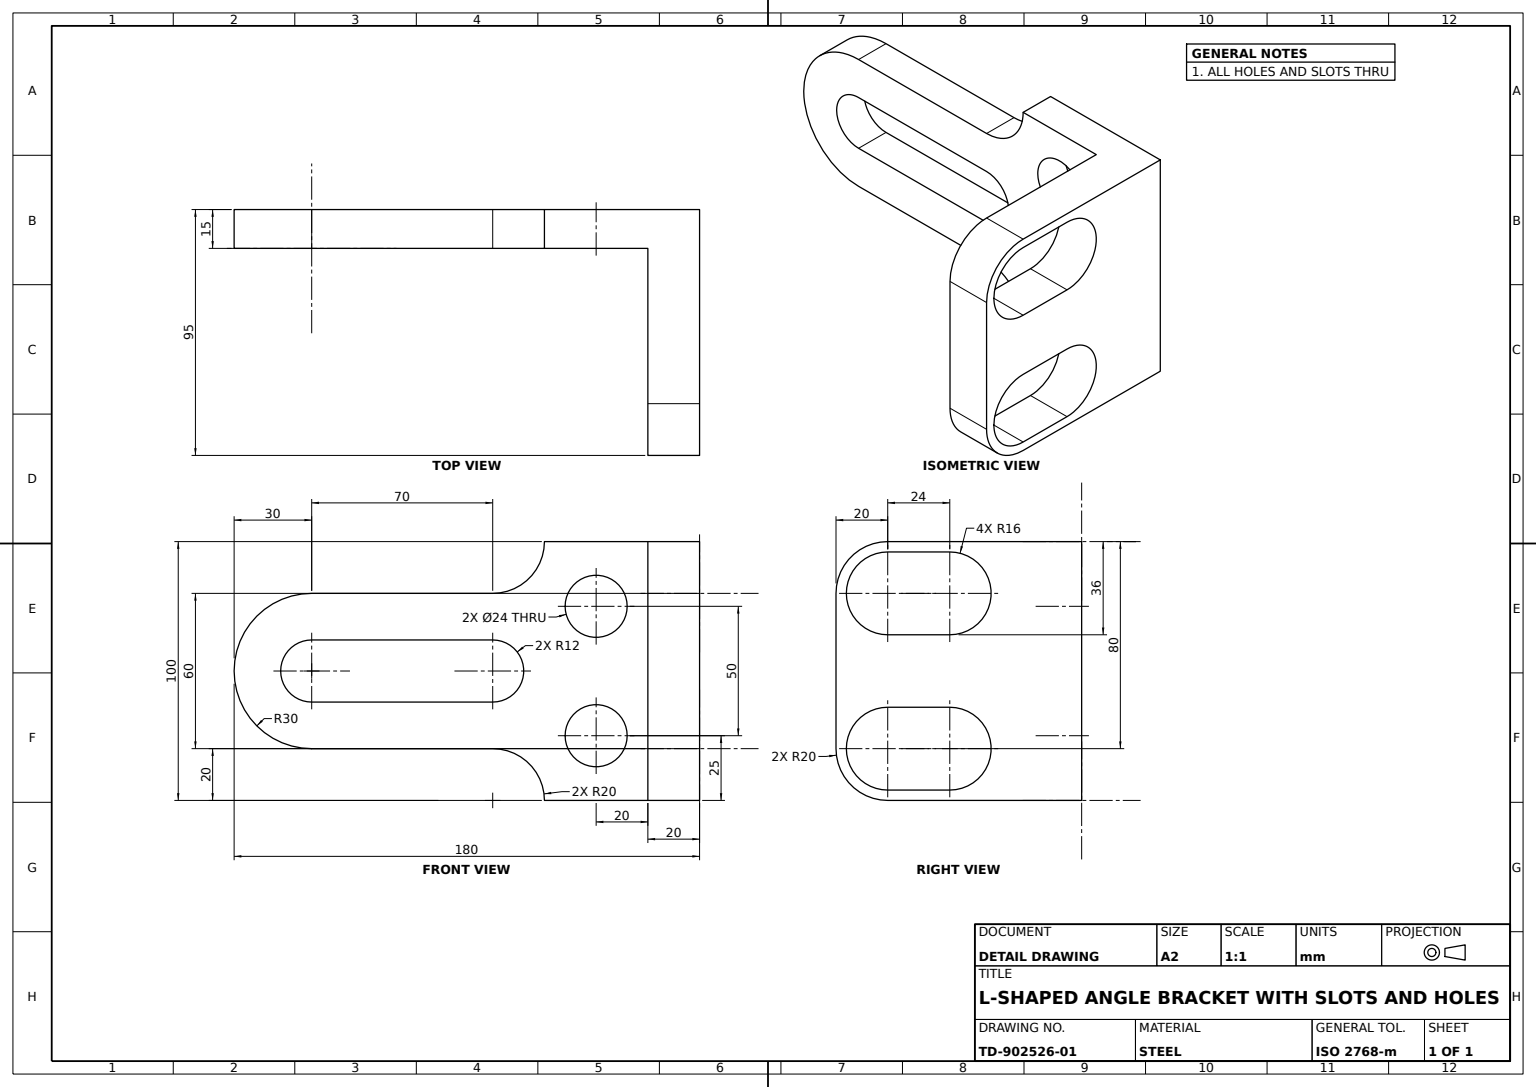
SolidWorks part; units mm, degrees
material "Plain Carbon Steel"
ref_plane "Front Plane" through (0, 0, 0) normal (0, 0, 1) x (1, 0, 0)
ref_plane "Top Plane" through (0, 0, 0) normal (0, 1, 0) x (1, 0, 0)
ref_plane "Right Plane" through (0, 0, 0) normal (1, 0, 0) x (0, 0, -1)
sketch "Base Block Sketch" plane through (0, 0, 0) normal (0, 0, 1) x (1, 0, 0)
  line L0 (0, 0) -> (60, 0)
  line L1 (80, 20) -> (80, 80)
  line L2 (60, 100) -> (0, 100)
  line L3 (0, 100) -> (0, 0)
  arc A0 (60, 0) -> (80, 20) centre (60, 20) ccw
  arc A1 (60, 100) -> (80, 80) centre (60, 80) cw
  dimension "D1" = 20
  dimension "D2" = 80
extrude "Base Block" add sketch "Base Block Sketch" along normal blind 20
sketch "Upright Plate Sketch" plane through (0, 0, 0) normal (-1, 0, 0) x (0, 0, 1)
  line L0 (20, 0) -> (60, 0)
  line L1 (60, 0) -> (60, 100)
  line L2 (60, 100) -> (0, 100)
  line L3 (0, 100) -> (0, 0)
  line L4 (0, 0) -> (20, 0)
  line L5 (0, 100) -> (0, 0) construction
  dimension "D1" = 60
extrude "Upright Plate" add sketch "Upright Plate Sketch" along normal blind 15
sketch "Slotted Arm Sketch" plane through (-15, 0, 0) normal (-1, 0, 0) x (0, 0, 1)
  line L0 (150, 80) -> (80, 80)
  line L2 (150, 20) -> (80, 20)
  line L3 (80, 62) -> (150, 62)
  line L5 (150, 38) -> (80, 38)
  line L6 (60, 100) -> (60, 0)
  line L7 (60, 0) -> (60, 100) construction
  arc A0 (80, 62) -> (80, 38) centre (80, 50) ccw
  arc A1 (150, 38) -> (150, 62) centre (150, 50) ccw
  arc A2 (150, 20) -> (150, 80) centre (150, 50) ccw
  arc A3 (80, 80) -> (60, 100) centre (80, 100) cw
  arc A4 (80, 20) -> (60, 0) centre (80, 0) ccw
  dimension "D1" = 12
  dimension "D2" = 30
  dimension "D3" = 90
extrude "Slotted Arm" add sketch "Slotted Arm Sketch" against normal blind 15
sketch "Holes 2x Sketch" plane through (0, 0, 0) normal (1, 0, 0) x (0, 0, -1)
  line L0 (-20, 100) -> (-20, 0) construction
  line L1 (-20, 20) -> (-20, 0) construction
  line L2 (-60, 100) -> (-20, 100) construction
  line L3 (-20, 0) -> (-60, 0) construction
  circle A0 centre (-40, 75) radius 12
  circle A1 centre (-40, 25) radius 12
  dimension "D1" = 20
  dimension "D5" = 24
  dimension "D2" = 20
  dimension "D3" = 25
  dimension "D4" = 25
extrude "Holes 2x" cut sketch "Holes 2x Sketch" against normal blind 15
sketch "Slots 2x Sketch" plane through (0, 0, 20) normal (0, 0, 1) x (1, 0, 0)
  line L0 (0, 100) -> (0, 0) construction
  line L1 (36, 96) -> (60, 96)
  line L2 (36, 36) -> (60, 36)
  line L4 (60, 4) -> (36, 4)
  line L5 (60, 64) -> (36, 64)
  arc A0 (60, 64) -> (60, 96) centre (60, 80) ccw
  arc A1 (60, 4) -> (60, 36) centre (60, 20) ccw
  arc A2 (36, 96) -> (36, 64) centre (36, 80) ccw
  arc A3 (36, 36) -> (36, 4) centre (36, 20) ccw
  dimension "D1" = 16
  dimension "D2" = 36
extrude "Slots 2x" cut sketch "Slots 2x Sketch" against normal blind 20
